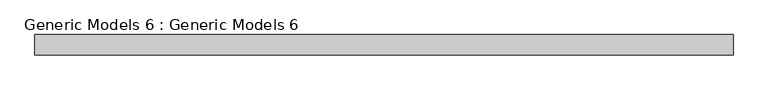
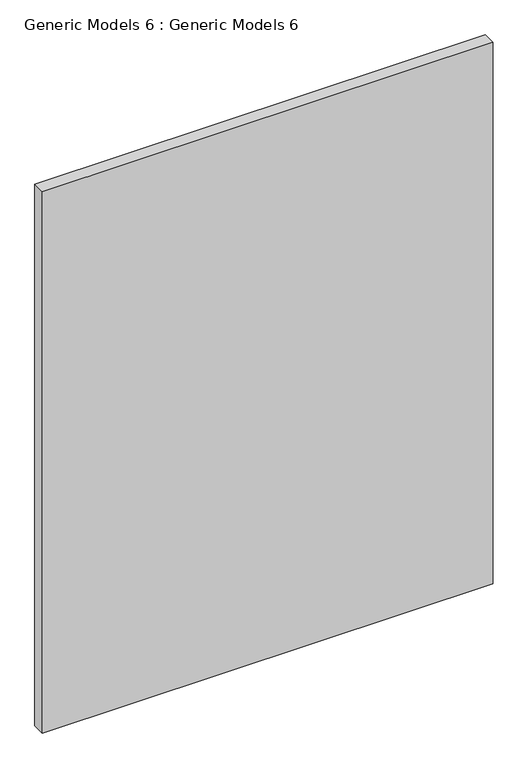
"""IFC4 building model written with IfcOpenShell, lengths in millimetres: proxy geometry, Generic Models 6 : Generic Models 6."""

from ifc_helpers import new_model, si_unit, origin, origin_with_axes, place, context, project, spatial, polyline, outline, extrude, source, transform, mapped, element, save


def generic_models_6_generic_models_6_d33aa09a(model_context):
    return source(origin(), model_context, "Body", "SweptSolid", [
        extrude(outline(polyline([(589.554407, -4187.674389), (-2052.0455733, -4187.674389), (-2052.0455733, -4111.474389), (589.554407, -4111.474389), (589.554407, -4187.674389)])), origin_with_axes(), (0.0, 0.0, 1.0), 3352.8),
    ])


if __name__ == "__main__":
    model = new_model("IFC4")
    model_context = context("Model", 3, world=origin())
    ifc_project = project(units=[si_unit("LENGTHUNIT", "METRE", prefix="MILLI")], contexts=[model_context])
    site = spatial("IfcSite", under=ifc_project)
    building = spatial("IfcBuilding", under=site)
    placement = place(None, origin())
    generic_models_6_generic_models_6_shape = generic_models_6_generic_models_6_d33aa09a(model_context)
    element("IfcBuildingElementProxy", 1, Name="Generic Models 6 : Generic Models 6", ObjectType="Generic Models 6 : Generic Models 6", at=placement, inside=building, context=model_context, shape_type="MappedRepresentation", body=[
        mapped(generic_models_6_generic_models_6_shape, transform((0.0, 0.0, 0.0), x_axis=(1.0, 0.0, 0.0), y_axis=(0.0, 1.0, 0.0), z_axis=(0.0, 0.0, 1.0))),
    ])
    save(model, "model.ifc")

# Revit data of these elements
# Element 1 (IfcBuildingElementProxy, "Generic Models 6 : Generic Models 6")
#   Materials on its faces: "LIGHT GREY WHITE"
# Materials
#   "LIGHT GREY WHITE": class "Generic", colour RGB 120 120 120, transparency 0, Cost = 0
